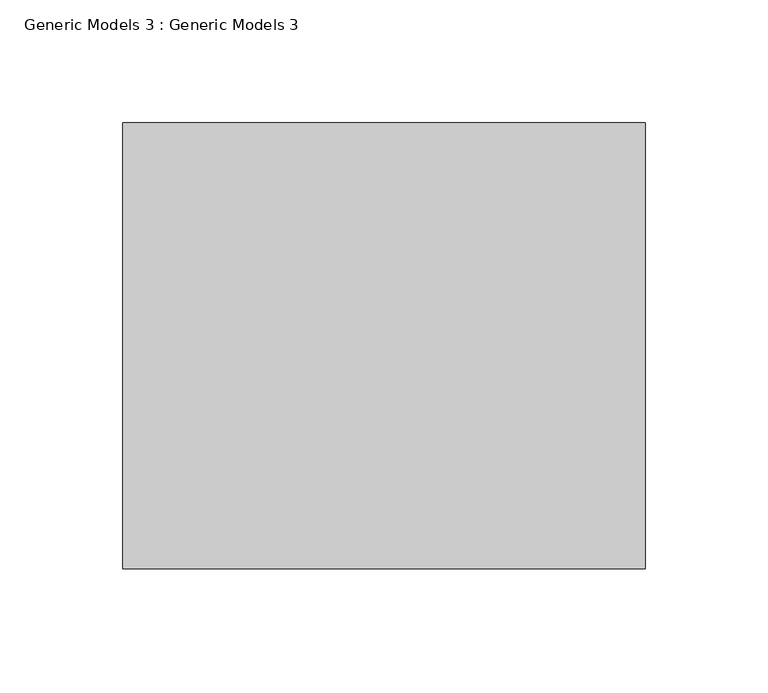
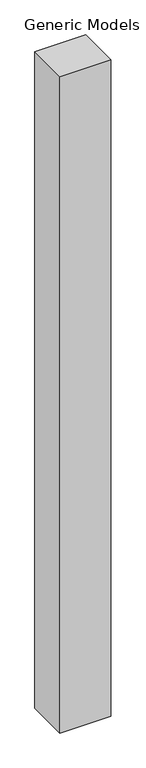
"""IFC4 building model written with IfcOpenShell, lengths in millimetres: proxy geometry, Generic Models 3 : Generic Models 3."""

from ifc_helpers import new_model, si_unit, frame, origin, place, context, project, spatial, polyline, outline, extrude, source, transform, mapped, element, save


def generic_models_3_generic_models_3_3f4cf848(model_context):
    return source(origin(), model_context, "Body", "SweptSolid", [
        extrude(outline(polyline([(-6117.2767684, -15311.3787587), (-6330.1189768, -15311.3787587), (-6330.1189768, -15129.6591816), (-6117.2767684, -15129.6591816), (-6117.2767684, -15311.3787587)])), frame((0.0, 0.0, 3352.8), z_axis=(0.0, 0.0, 1.0), x_axis=(1.0, 0.0, 0.0)), (0.0, 0.0, 1.0), 2909.2193651),
    ])


if __name__ == "__main__":
    model = new_model("IFC4")
    model_context = context("Model", 3, world=origin())
    ifc_project = project(units=[si_unit("LENGTHUNIT", "METRE", prefix="MILLI")], contexts=[model_context])
    site = spatial("IfcSite", under=ifc_project)
    building = spatial("IfcBuilding", under=site)
    placement = place(None, origin())
    generic_models_3_generic_models_3_shape = generic_models_3_generic_models_3_3f4cf848(model_context)
    element("IfcBuildingElementProxy", 1, Name="Generic Models 3 : Generic Models 3", ObjectType="Generic Models 3 : Generic Models 3", at=placement, inside=building, context=model_context, shape_type="MappedRepresentation", body=[
        mapped(generic_models_3_generic_models_3_shape, transform((0.0, 0.0, 0.0), x_axis=(1.0, 0.0, 0.0), y_axis=(0.0, 1.0, 0.0), z_axis=(0.0, 0.0, 1.0))),
    ])
    save(model, "model.ifc")
